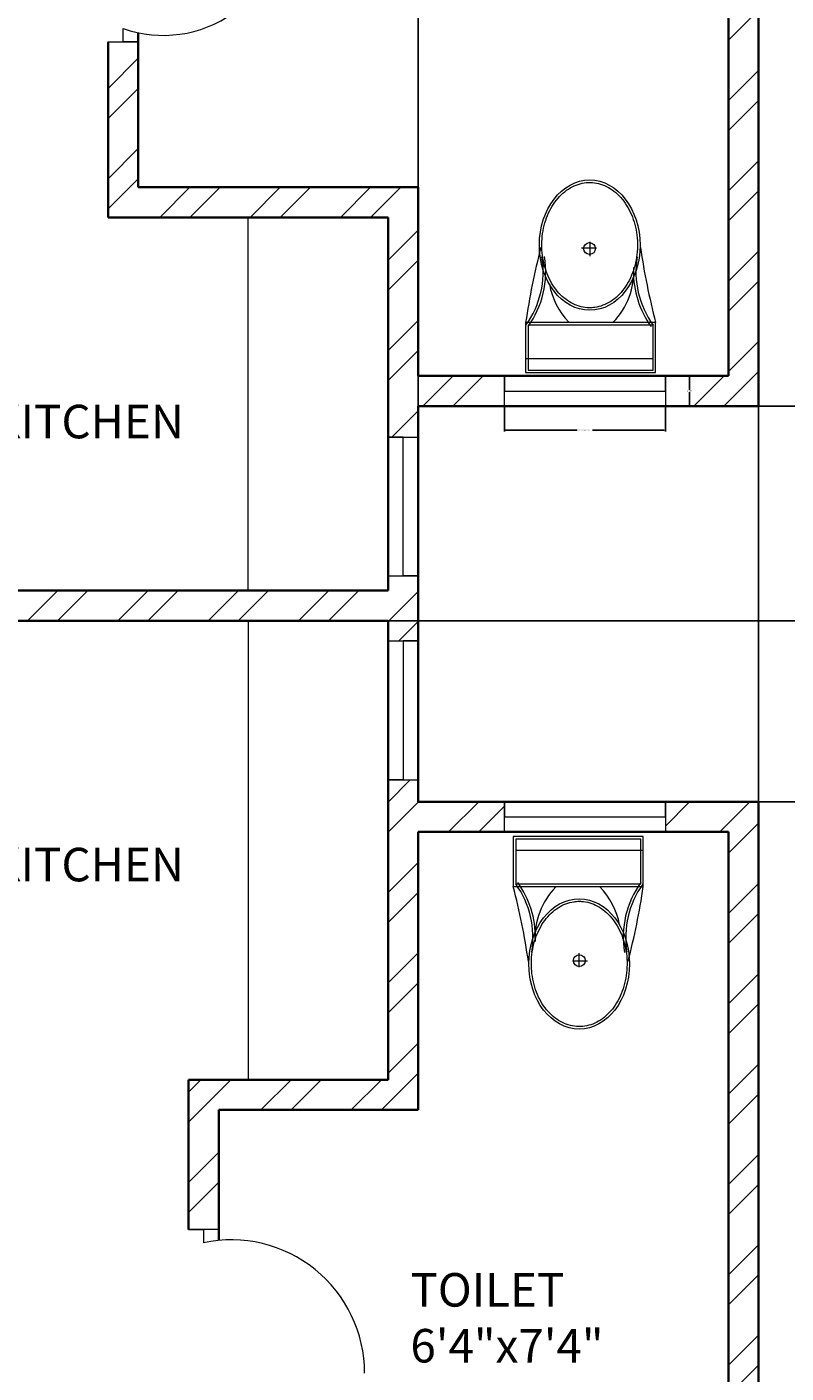
# Model space of a CAD drawing. Units: inches. Extents: x 2165 to 3042, y 1626 to 2968.
# Tile 8 of 11: x 2776 to 2889, y 1990 to 2191. Entities that reach past the tile are written whole.
import ezdxf

# ---------------------------------------------------------------- set-up
doc = ezdxf.new("R2010")
doc.units = ezdxf.units.IN
for name, color, linetype, lineweight in [('A-ANNO-DIMS', 2, 'Continuous', 18), ('A-AREA-IDEN', 7, 'Continuous', 18), ('A-DOOR', 3, 'Continuous', 18), ('A-FLOR-CASE', 8, 'Continuous', 18), ('A-FLOR-FIXT', 9, 'Continuous', 18), ('A-GLAZ', 4, 'Continuous', 18), ('A-WALL', 7, 'Continuous', 35), ('A-WALL-PATT', 252, 'Continuous', 13)]:
    doc.layers.add(name, color=color, linetype=linetype, lineweight=lineweight)
doc.styles.get("Standard").update_dxf_attribs({"font": 'arial.ttf'})
doc.dimstyles.get("Standard").update_dxf_attribs({"dimtxt": 0.18, "dimasz": 0.18, "dimexe": 0.18, "dimexo": 0.0625, "dimgap": 0.09, "dimtad": 0, "dimtih": 1, "dimtoh": 1, "dimdec": 4, "dimzin": 0, "dimdsep": 46, "dimtxsty": 'Standard', "dimcen": 0.09, "dimadec": 0, "dimazin": 0, "dimtfac": 1, "dimtdec": 4, "dimtofl": 0, "dimtmove": 0, "dimatfit": 3, "dimfxl": 1, "dimtolj": 1, "dimtzin": 0, "dimarcsym": 0})

# ---------------------------------------------------------------- blocks, each defined once
blk = doc.blocks.new('A$C31115884')
for p, q in [((283.1, 497.7), (223.4, 497.7)), ((257.5, 466.4), (257.5, 523.2)), ((0, 200), (0, 0)), ((520, 200), (0, 200)), ((10, 190), (10, 10)), ((510, 190), (10, 190)), ((510, 10), (510, 190)), ((520, 0), (520, 200)), ((510, 54.5), (0, 54.5)), ((10, 10), (510, 10)), ((0, 0), (520, 0))]:
    blk.add_line(p, q)
blk.add_circle((255.6, 496.4), 23.6)
for centre, radius, start, end in [((2777.7, -204.6), 2807, 165.4549, 171.7133), ((3237, 905), 2807, 188.2867, 194.5451), ((-294.5, 403.3), 364.7, 324.2091, 9.3499), ((-294.5, 403.3), 374.7, 324.2091, 9.3499), ((805.8, 403.3), 364.7, 170.6501, 215.7909), ((139.5, 406.2), 293.5, 315.8436, 2.6563), ((805.8, 403.3), 374.7, 179.2036, 215.7909), ((383.6, 406.2), 293.5, 190.2774, 224.1564)]:
    blk.add_arc(centre, radius, start, end)
blk.add_ellipse((256.2, 509.9), major_axis=(0, -260.7), ratio=0.772727)
blk.add_open_spline([(256.2, 259.2), (263.1, 259.2), (270, 259.7), (287.8, 262.3), (298.7, 265.1), (319.9, 273.1), (330.2, 278.4), (350.1, 291.1), (359.7, 298.7), (377.7, 315.9), (386.2, 325.5), (401.7, 346.6), (408.8, 358.1), (421.3, 382.5), (426.8, 395.5), (435.9, 422.4), (439.5, 436.4), (444.8, 465.1), (446.5, 479.7), (447.9, 509.2), (447.6, 524), (445, 553.3), (442.7, 567.8), (436.3, 596), (432.1, 609.7), (421.9, 636), (416, 648.6), (402.5, 672.1), (395, 683), (378.6, 703), (369.8, 712.1), (351.1, 728), (341.3, 734.8), (320.9, 746.2), (310.4, 750.7), (288.9, 757.3), (278, 759.4), (256, 761), (245, 760.6), (223.1, 757.2), (212.3, 754.3), (191.1, 746.1), (180.8, 740.7), (160.9, 727.8), (151.4, 720.1), (133.5, 702.7), (125.1, 693), (109.6, 671.7), (102.6, 660.2), (90.2, 635.7), (84.9, 622.7), (76, 595.6), (72.4, 581.6), (67.2, 552.9), (65.6, 538.2), (64.4, 508.8), (64.8, 494), (67.5, 464.7), (69.9, 450.2), (76.6, 422), (80.8, 408.3), (91.1, 382.2), (97.2, 369.7), (110.8, 346.3), (118.4, 335.4), (134.8, 315.6), (143.7, 306.7), (162.4, 290.9), (172.3, 284.2), (192.8, 273), (203.3, 268.6), (224.8, 262.2), (235.8, 260.2), (249.9, 259.3), (253, 259.2), (256.2, 259.2)], degree=3, knots=[0, 0, 0, 0, 0.110105, 0.110105, 0.285049, 0.285049, 0.459994, 0.459994, 0.634938, 0.634938, 0.809882, 0.809882, 0.984827, 0.984827, 1.159771, 1.159771, 1.334715, 1.334715, 1.50966, 1.50966, 1.684604, 1.684604, 1.859549, 1.859549, 2.034493, 2.034493, 2.209437, 2.209437, 2.384382, 2.384382, 2.559326, 2.559326, 2.73427, 2.73427, 2.909215, 2.909215, 3.084159, 3.084159, 3.259103, 3.259103, 3.434048, 3.434048, 3.608992, 3.608992, 3.783936, 3.783936, 3.958881, 3.958881, 4.133825, 4.133825, 4.30877, 4.30877, 4.483714, 4.483714, 4.658658, 4.658658, 4.833603, 4.833603, 5.008547, 5.008547, 5.183491, 5.183491, 5.358436, 5.358436, 5.53338, 5.53338, 5.708324, 5.708324, 5.883269, 5.883269, 6.058213, 6.058213, 6.233158, 6.233158, 6.283185, 6.283185, 6.283185, 6.283185])
blk = doc.blocks.new('WIN-24')
for p, q in [((0, 0), (0, 4.5)), ((0, 4.5), (0, 2.25)), ((24, 2.25), (24, 4.5)), ((24, 4.5), (24, 0)), ((0, 2.25), (24, 2.25))]:
    blk.add_line(p, q)
blk = doc.blocks.new('*D28')
at = {"layer": 'A-ANNO-DIMS', "color": 0, "lineweight": -2, "transparency": 16777216}
for p, q in [((2847.2, 2134.52), (2847.2, 2130.8)), ((2871.2, 2134.52), (2871.2, 2130.8)), ((2847.38, 2130.98), (2858.05, 2130.98)), ((2871.02, 2130.98), (2860.36, 2130.98))]:
    blk.add_line(p, q, dxfattribs=at)
at = {"layer": 'A-ANNO-DIMS', "color": 0, "transparency": 16777216}
for points in [[(2847.38, 2131.01), (2847.38, 2130.95), (2847.2, 2130.98)], [(2871.02, 2131.01), (2871.02, 2130.95), (2871.2, 2130.98)]]:
    blk.add_solid(points, dxfattribs=at)
at = {"layer": 'Defpoints', "color": 0, "transparency": 16777216}
for p in [(2847.2, 2134.58), (2871.2, 2134.58), (2871.2, 2130.98)]:
    blk.add_point(p, dxfattribs=at)
at = {"layer": 'A-ANNO-DIMS', "color": 0, "transparency": 16777216, "insert": (2859.2, 2130.98), "char_height": 0.18, "attachment_point": 5}
blk.add_mtext('\\A1;WC SASH 24 TYP.', dxfattribs=at)
blk = doc.blocks.new('*D29')
at = {"layer": 'A-ANNO-DIMS', "color": 0, "lineweight": -2, "transparency": 16777216}
for p, q in [((2871.27, 2139.08), (2874.98, 2139.08)), ((2874.8, 2138.9), (2874.8, 2137.01)), ((2874.8, 2134.76), (2874.8, 2136.65)), ((2871.27, 2134.58), (2874.98, 2134.58))]:
    blk.add_line(p, q, dxfattribs=at)
at = {"layer": 'A-ANNO-DIMS', "color": 0, "transparency": 16777216}
for points in [[(2874.77, 2138.9), (2874.83, 2138.9), (2874.8, 2139.08)], [(2874.77, 2134.76), (2874.83, 2134.76), (2874.8, 2134.58)]]:
    blk.add_solid(points, dxfattribs=at)
at = {"layer": 'Defpoints', "color": 0, "transparency": 16777216}
for p in [(2871.2, 2139.08), (2874.8, 2139.08), (2871.2, 2134.58)]:
    blk.add_point(p, dxfattribs=at)
at = {"layer": 'A-ANNO-DIMS', "color": 0, "transparency": 16777216, "insert": (2874.8, 2136.83), "char_height": 0.18, "attachment_point": 5}
blk.add_mtext('\\A1;5 TYP.', dxfattribs=at)
blk = doc.blocks.new('*D58')
at = {"layer": 'A-ANNO-DIMS', "color": 0, "lineweight": -2, "transparency": 16777216}
for p, q in [((2885.17, 2075.58), (2919.58, 2075.58)), ((2919.4, 2075.4), (2919.4, 2027.26)), ((2919.4, 1978.76), (2919.4, 2026.9)), ((2880.67, 1978.58), (2919.58, 1978.58))]:
    blk.add_line(p, q, dxfattribs=at)
at = {"layer": 'A-ANNO-DIMS', "color": 0, "transparency": 16777216}
for points in [[(2919.37, 2075.4), (2919.43, 2075.4), (2919.4, 2075.58)], [(2919.37, 1978.76), (2919.43, 1978.76), (2919.4, 1978.58)]]:
    blk.add_solid(points, dxfattribs=at)
at = {"layer": 'Defpoints', "color": 0, "transparency": 16777216}
for p in [(2885.1, 2075.58), (2919.4, 2075.58), (2880.6, 1978.58)]:
    blk.add_point(p, dxfattribs=at)
at = {"layer": 'A-ANNO-DIMS', "color": 0, "transparency": 16777216, "insert": (2919.4, 2027.08), "char_height": 0.18, "attachment_point": 5}
blk.add_mtext('\\A1;97', dxfattribs=at)
blk = doc.blocks.new('*D59')
at = {"layer": 'A-ANNO-DIMS', "color": 0, "lineweight": -2, "transparency": 16777216}
for p, q in [((2829.92, 2102.58), (2919.58, 2102.58)), ((2919.4, 2102.4), (2919.4, 2089.26)), ((2919.4, 2075.76), (2919.4, 2088.9)), ((2885.17, 2075.58), (2919.58, 2075.58))]:
    blk.add_line(p, q, dxfattribs=at)
at = {"layer": 'A-ANNO-DIMS', "color": 0, "transparency": 16777216}
for points in [[(2919.37, 2102.4), (2919.43, 2102.4), (2919.4, 2102.58)], [(2919.37, 2075.76), (2919.43, 2075.76), (2919.4, 2075.58)]]:
    blk.add_solid(points, dxfattribs=at)
at = {"layer": 'Defpoints', "color": 0, "transparency": 16777216}
for p in [(2829.85, 2102.58), (2919.4, 2102.58), (2885.1, 2075.58)]:
    blk.add_point(p, dxfattribs=at)
at = {"layer": 'A-ANNO-DIMS', "color": 0, "transparency": 16777216, "insert": (2919.4, 2089.08), "char_height": 0.18, "attachment_point": 5}
blk.add_mtext('\\A1;27', dxfattribs=at)
blk = doc.blocks.new('*D60')
at = {"layer": 'A-ANNO-DIMS', "color": 0, "lineweight": -2, "transparency": 16777216}
for p, q in [((2885.17, 2134.58), (2919.58, 2134.58)), ((2919.4, 2134.4), (2919.4, 2118.76)), ((2919.4, 2102.76), (2919.4, 2118.4)), ((2829.92, 2102.58), (2919.58, 2102.58))]:
    blk.add_line(p, q, dxfattribs=at)
at = {"layer": 'A-ANNO-DIMS', "color": 0, "transparency": 16777216}
for points in [[(2919.37, 2134.4), (2919.43, 2134.4), (2919.4, 2134.58)], [(2919.37, 2102.76), (2919.43, 2102.76), (2919.4, 2102.58)]]:
    blk.add_solid(points, dxfattribs=at)
at = {"layer": 'Defpoints', "color": 0, "transparency": 16777216}
for p in [(2885.1, 2134.58), (2919.4, 2134.58), (2829.85, 2102.58)]:
    blk.add_point(p, dxfattribs=at)
at = {"layer": 'A-ANNO-DIMS', "color": 0, "transparency": 16777216, "insert": (2919.4, 2118.58), "char_height": 0.18, "attachment_point": 5}
blk.add_mtext('\\A1;32', dxfattribs=at)
blk = doc.blocks.new('*D61')
at = {"layer": 'A-ANNO-DIMS', "color": 0, "lineweight": -2, "transparency": 16777216}
for p, q in [((2880.67, 2215.08), (2919.58, 2215.08)), ((2919.4, 2214.9), (2919.4, 2175.01)), ((2919.4, 2134.76), (2919.4, 2174.65)), ((2885.17, 2134.58), (2919.58, 2134.58))]:
    blk.add_line(p, q, dxfattribs=at)
at = {"layer": 'A-ANNO-DIMS', "color": 0, "transparency": 16777216}
for points in [[(2919.37, 2214.9), (2919.43, 2214.9), (2919.4, 2215.08)], [(2919.37, 2134.76), (2919.43, 2134.76), (2919.4, 2134.58)]]:
    blk.add_solid(points, dxfattribs=at)
at = {"layer": 'Defpoints', "color": 0, "transparency": 16777216}
for p in [(2880.6, 2215.08), (2919.4, 2215.08), (2885.1, 2134.58)]:
    blk.add_point(p, dxfattribs=at)
at = {"layer": 'A-ANNO-DIMS', "color": 0, "transparency": 16777216, "insert": (2919.4, 2174.83), "char_height": 0.18, "attachment_point": 5}
blk.add_mtext('\\A1;80.5', dxfattribs=at)
blk = doc.blocks.new('*D63')
at = {"layer": 'A-ANNO-DIMS', "color": 0, "lineweight": -2, "transparency": 16777216}
for p, q in [((2834.35, 2075.64), (2834.35, 2398.06)), ((2834.53, 2397.88), (2859.34, 2397.88)), ((2884.92, 2397.88), (2860.12, 2397.88)), ((2885.1, 2075.64), (2885.1, 2398.06))]:
    blk.add_line(p, q, dxfattribs=at)
at = {"layer": 'A-ANNO-DIMS', "color": 0, "transparency": 16777216}
for points in [[(2834.53, 2397.91), (2834.53, 2397.85), (2834.35, 2397.88)], [(2884.92, 2397.91), (2884.92, 2397.85), (2885.1, 2397.88)]]:
    blk.add_solid(points, dxfattribs=at)
at = {"layer": 'Defpoints', "color": 0, "transparency": 16777216}
for p in [(2885.1, 2397.88), (2834.35, 2075.58), (2885.1, 2075.58)]:
    blk.add_point(p, dxfattribs=at)
at = {"layer": 'A-ANNO-DIMS', "color": 0, "transparency": 16777216, "insert": (2859.73, 2397.88), "char_height": 0.18, "attachment_point": 5}
blk.add_mtext('\\A1;50.75', dxfattribs=at)

msp = doc.modelspace()

# ---------------------------------------------------------------- hatches: boundary and pattern name
at = {"layer": 'A-WALL-PATT'}
h = msp.add_hatch(dxfattribs=at)
h.set_pattern_fill('ANSI32', color=256)
h.paths.add_polyline_path([(2406.4931, 2332.0783), (2286.6045, 2332.0783), (2286.6045, 2310.967), (2288.8545, 2310.967), (2291.1045, 2310.967), (2291.1045, 2327.5783), (2406.4931, 2327.5783), (2406.4931, 2329.8283)])
h.paths.add_polyline_path([(2439.6045, 2327.5783), (2444.9584, 2327.5783), (2444.9584, 2332.0783), (2430.2901, 2332.0783), (2430.2901, 2329.8283), (2430.2901, 2327.5783), (2435.1045, 2327.5783), (2435.1045, 2219.5783), (2431.0902, 2219.5783), (2431.0902, 2215.0783), (2435.1045, 2215.0783), (2444.1108, 2215.0783), (2444.1108, 2217.3283), (2444.1108, 2219.5783), (2439.6045, 2219.5783)])
h.paths.add_polyline_path([(2497.5418, 2329.8283), (2497.5418, 2332.0783), (2470.1978, 2332.0783), (2470.1978, 2327.5783), (2497.5418, 2327.5783)])
h.paths.add_polyline_path([(2617.9543, 2332.0783), (2557.5418, 2332.0783), (2557.5418, 2327.5783), (2583.6045, 2327.5783), (2583.6045, 2219.5783), (2474.0523, 2219.5783), (2474.0523, 2215.0783), (2583.6045, 2215.0783), (2583.6045, 2107.0783), (2579.3609, 2107.0783), (2579.3609, 2102.5783), (2588.1045, 2102.5783), (2593.5283, 2102.5783), (2593.5283, 2104.8283), (2593.5283, 2107.0783), (2588.1045, 2107.0783), (2588.1045, 2215.0783), (2691.2325, 2215.0783), (2691.2325, 2217.3283), (2691.2325, 2219.5783), (2588.1045, 2219.5783), (2588.1045, 2327.5783), (2617.9543, 2327.5783)])
h.paths.add_polyline_path([(2702.4444, 2329.8283), (2702.4444, 2332.0783), (2677.9543, 2332.0783), (2677.9543, 2327.5783), (2702.4444, 2327.5783)])
h.paths.add_polyline_path([(2736.6045, 2327.5783), (2742.5161, 2327.5783), (2742.5161, 2329.8283), (2742.5161, 2332.0783), (2727.7639, 2332.0783), (2727.7639, 2329.8283), (2727.7639, 2327.5783), (2732.1045, 2327.5783), (2732.1045, 2219.5783), (2726.4404, 2219.5783), (2726.4404, 2215.0783), (2732.1045, 2215.0783), (2742.7291, 2215.0783), (2742.7291, 2217.3283), (2742.7291, 2219.5783), (2736.6045, 2219.5783)])
h.paths.add_polyline_path([(2885.1045, 2332.0783), (2768.4887, 2332.0783), (2768.4887, 2327.5783), (2784.6045, 2327.5783), (2880.6045, 2327.5783), (2880.6045, 2310.967), (2885.1045, 2310.967)])
h.paths.add_polyline_path([(2885.1045, 2250.967), (2880.6045, 2250.967), (2880.6045, 2219.5783), (2776.5755, 2219.5783), (2776.5755, 2215.0783), (2788.1045, 2215.0783), (2788.1045, 2209.8634), (2790.3545, 2209.8634), (2792.6045, 2209.8634), (2792.6045, 2215.0783), (2880.6045, 2215.0783), (2880.6045, 2139.0783), (2871.2037, 2139.0783), (2871.2037, 2134.5783), (2885.1045, 2134.5783)])
h.paths.add_polyline_path([(2545.013, 2107.0783), (2474.0523, 2107.0783), (2291.1045, 2107.0783), (2291.1045, 2102.5783), (2535.6045, 2102.5783), (2535.6045, 2096.8046), (2537.8545, 2096.8046), (2540.1045, 2096.8046), (2540.1045, 2102.5783), (2545.013, 2102.5783), (2545.013, 2104.8283)])
h.paths.add_polyline_path([(2397.7297, 2217.3283), (2397.7297, 2219.5783), (2291.1045, 2219.5783), (2291.1045, 2250.967), (2286.6045, 2250.967), (2286.6045, 2206.1346), (2288.8545, 2206.1346), (2291.1045, 2206.1346), (2291.1045, 2215.0783), (2367.1045, 2215.0783), (2367.1045, 2212.2868), (2371.6045, 2212.2868), (2371.6045, 2215.0783), (2397.7297, 2215.0783)])
h.paths.add_polyline_path([(2291.1045, 1978.5783), (2367.1045, 1978.5783), (2371.6045, 1978.5783), (2373.2641, 1978.5783), (2374.4883, 1978.5783), (2374.4883, 1980.8283), (2374.4883, 1983.0783), (2371.6045, 1983.0783), (2371.6045, 1986.964), (2369.9051, 1986.964), (2369.3545, 1986.964), (2367.1045, 1986.964), (2367.1045, 1983.0783), (2291.1045, 1983.0783), (2291.1045, 2001.1808), (2286.6045, 2001.1808), (2286.6045, 1947.0203), (2288.8545, 1947.0203), (2291.1045, 1947.0203)])
h.paths.add_polyline_path([(2291.1045, 1887.0203), (2286.6045, 1887.0203), (2286.6045, 1842.0783), (2381.2561, 1842.0783), (2381.2561, 1844.3283), (2381.2561, 1846.5783), (2363.1045, 1846.5783), (2291.1045, 1846.5783)])
h.paths.add_polyline_path([(2415.6045, 1978.5783), (2421.1681, 1978.5783), (2421.1681, 1983.0783), (2415.6045, 1983.0783), (2406.5227, 1983.0783), (2406.5227, 1980.8283), (2406.5227, 1978.5783), (2411.1045, 1978.5783), (2411.1045, 1846.5783), (2406.7549, 1846.5783), (2406.7549, 1842.0783), (2419.2885, 1842.0783), (2419.2885, 1844.3283), (2419.2885, 1846.5783), (2415.6045, 1846.5783)])
h.paths.add_polyline_path([(2586.6045, 1982.779), (2586.6045, 1991.5911), (2582.1045, 1991.5911), (2582.1045, 1982.779), (2540.1045, 1982.779), (2540.1045, 2036.779), (2582.1045, 2036.779), (2582.1045, 2027.6051), (2586.6045, 2027.6051), (2586.6045, 2041.279), (2582.1045, 2041.279), (2540.1045, 2041.279), (2540.1045, 2063.9064), (2537.8545, 2063.9064), (2535.6045, 2063.9064), (2535.6045, 1983.0783), (2455.068, 1983.0783), (2455.068, 1978.5783), (2535.6045, 1978.5783), (2535.6045, 1846.5783), (2522.622, 1846.5783), (2522.622, 1842.0783), (2535.6045, 1842.0783), (2535.6045, 1806.0783), (2535.6045, 1801.5783), (2556.726, 1801.5783), (2556.726, 1803.8283), (2556.726, 1806.0783), (2540.1045, 1806.0783), (2540.1045, 1842.0783), (2540.1045, 1846.5783), (2540.1045, 1978.279), (2586.6045, 1978.279)])
h.paths.add_polyline_path([(2636.1045, 1978.5783), (2717.6642, 1978.5783), (2717.6642, 1980.8283), (2717.6642, 1983.0783), (2636.1045, 1983.0783), (2636.1045, 2063.9064), (2633.8545, 2063.9064), (2631.6045, 2063.9064), (2631.6045, 1846.5783), (2631.6045, 1842.0783), (2631.6045, 1806.0783), (2604.726, 1806.0783), (2604.726, 1801.5783), (2636.1045, 1801.5783), (2636.1045, 1842.0783), (2644.3411, 1842.0783), (2644.3411, 1844.3283), (2644.3411, 1846.5783), (2636.1045, 1846.5783)])
h.paths.add_polyline_path([(2760.6045, 1978.5783), (2764.9931, 1978.5783), (2764.9931, 1983.0783), (2750.4727, 1983.0783), (2750.4727, 1980.8283), (2750.4727, 1978.5783), (2756.1045, 1978.5783), (2756.1045, 1846.5783), (2749.4543, 1846.5783), (2749.4543, 1842.0783), (2765.1894, 1842.0783), (2765.1894, 1846.5783), (2760.6045, 1846.5783)])
h.paths.add_polyline_path([(2880.6045, 1983.0783), (2804.6045, 1983.0783), (2804.6045, 1988.3825), (2802.3545, 1988.3825), (2800.1045, 1988.3825), (2800.1045, 1983.0783), (2800.1045, 1978.5783), (2880.6045, 1978.5783)])
h.paths.add_polyline_path([(2885.1045, 2075.5783), (2871.2037, 2075.5783), (2871.2037, 2071.0783), (2880.6045, 2071.0783), (2880.6045, 1948.8144), (2885.1045, 1948.8144)])
h.paths.add_polyline_path([(2885.1045, 1888.8144), (2880.6045, 1888.8144), (2880.6045, 1846.5783), (2792.1167, 1846.5783), (2792.1167, 1842.0783), (2885.1045, 1842.0783)])
h.paths.add_polyline_path([(2724.4848, 1846.5783), (2708.1045, 1846.5783), (2692.3411, 1846.5783), (2692.3411, 1842.0783), (2724.4848, 1842.0783), (2724.4848, 1844.3283)])
h.paths.add_polyline_path([(2474.622, 1844.4672), (2474.622, 1846.5783), (2444.7417, 1846.5783), (2444.7417, 1842.0783), (2474.622, 1842.0783)])
h = msp.add_hatch(dxfattribs=at)
h.set_pattern_fill('ANSI32', color=256)
h.paths.add_polyline_path([(2834.3545, 2109.2607), (2832.1045, 2109.2607), (2829.8545, 2109.2607), (2829.8545, 2107.0783), (2788.1045, 2107.0783), (2627.8367, 2107.0783), (2627.8367, 2102.5783), (2631.6045, 2102.5783), (2631.6045, 2096.8046), (2636.1045, 2096.8046), (2636.1045, 2102.5783), (2788.1045, 2102.5783), (2829.8545, 2102.5783), (2829.8545, 2099.5599), (2834.3545, 2099.5599), (2834.3545, 2102.5783)])
h.paths.add_polyline_path([(2834.3545, 2162.7002), (2834.3545, 2167.2002), (2792.6045, 2167.2002), (2792.6045, 2188.8893), (2790.3545, 2188.8893), (2788.1045, 2188.8893), (2788.1045, 2162.7002), (2829.8545, 2162.7002), (2829.8545, 2134.5783), (2829.8545, 2129.9534), (2834.3545, 2129.9534), (2834.3545, 2134.5783), (2847.2037, 2134.5783), (2847.2037, 2139.0783), (2834.3545, 2139.0783)])
h.paths.add_polyline_path([(2834.3545, 2071.0783), (2847.2037, 2071.0783), (2847.2037, 2075.5783), (2834.3545, 2075.5783), (2834.3545, 2078.8214), (2829.8545, 2078.8214), (2829.8545, 2075.5783), (2829.8545, 2034.1177), (2800.1045, 2034.1177), (2800.1045, 2011.8162), (2802.3375, 2011.8162), (2804.6045, 2011.8162), (2804.6045, 2029.6177), (2834.3545, 2029.6177), (2834.3545, 2034.1177)])

# ---------------------------------------------------------------- linework, layer by layer
at = {"layer": 'A-DOOR'}
for p, q in [((2790.3545, 2188.8893), (2790.3545, 2190.8893)), ((2788.1045, 2188.8893), (2792.6045, 2188.8893)), ((2792.6045, 2188.8893), (2790.3545, 2188.8893)), ((2790.3545, 2188.8893), (2790.3545, 2188.8893)), ((2801.4524, 2011.8162), (2800.1045, 2011.8162)), ((2800.1045, 2011.8162), (2802.3375, 2011.8162)), ((2804.6045, 2011.8162), (2801.4524, 2011.8162)), ((2802.3375, 2011.8162), (2802.3375, 2009.8162))]:
    msp.add_line(p, q, dxfattribs=at)
for centre, radius, start, end in [((2796.3519, 2207.8634), 18.0025, 250.540061, 0), ((2806.4834, 1990.3825), 19.8711, 0, 102.042606)]:
    msp.add_arc(centre, radius, start, end, dxfattribs=at)
at = {"layer": 'A-FLOR-CASE'}
for p, q in [((2808.9795, 2107.0783), (2808.9795, 2162.7002)), ((2808.9795, 2102.5783), (2808.9795, 2034.1177))]:
    msp.add_line(p, q, dxfattribs=at)
at = {"layer": 'A-GLAZ'}
for p, q in [((2832.1045, 2129.9534), (2829.8545, 2129.9534)), ((2829.8545, 2129.9534), (2834.3545, 2129.9534)), ((2832.1045, 2109.2607), (2832.1045, 2129.9534)), ((2829.8545, 2109.2607), (2834.3545, 2109.2607)), ((2834.3545, 2109.2607), (2832.1045, 2109.2607)), ((2829.8545, 2099.5599), (2834.3545, 2099.5599)), ((2834.3545, 2099.5599), (2832.1045, 2099.5599)), ((2832.1045, 2099.5599), (2832.1045, 2078.8214)), ((2832.1045, 2078.8214), (2829.8545, 2078.8214)), ((2829.8545, 2078.8214), (2834.3545, 2078.8214))]:
    msp.add_line(p, q, dxfattribs=at)
at = {"layer": 'A-WALL'}
for p, q in [((2885.1045, 2332.0783), (2885.1045, 2134.5783)), ((2880.6045, 2215.0783), (2880.6045, 2139.0783)), ((2792.6045, 2190.2552), (2792.6045, 2167.2002)), ((2788.1045, 2188.8893), (2788.1045, 2162.7002)), ((2834.3545, 2167.2002), (2792.6045, 2167.2002)), ((2834.3545, 2162.7002), (2834.3545, 2167.2002)), ((2829.8545, 2162.7002), (2788.1045, 2162.7002)), ((2829.8545, 2134.5783), (2829.8545, 2162.7002)), ((2834.3545, 2139.0783), (2834.3545, 2162.7002)), ((2834.3545, 2139.0783), (2880.6045, 2139.0783)), ((2829.8545, 2107.0783), (2829.8545, 2134.5783)), ((2834.3545, 2134.5783), (2885.1045, 2134.5783)), ((2834.3545, 2134.5783), (2834.3545, 2075.5783)), ((2834.3545, 2134.5783), (2834.3545, 2134.5783)), ((2626.1408, 2107.0783), (2788.1045, 2107.0783)), ((2788.1045, 2107.0783), (2829.8545, 2107.0783)), ((2636.1045, 2102.5783), (2788.1045, 2102.5783)), ((2788.1045, 2102.5783), (2829.8545, 2102.5783)), ((2829.8545, 2075.5783), (2829.8545, 2102.5783)), ((2834.3545, 2102.5783), (2834.3545, 2075.5783)), ((2829.8545, 2075.5783), (2829.8545, 2034.1177)), ((2834.3545, 2075.5783), (2885.1045, 2075.5783)), ((2885.1045, 2075.5783), (2885.1045, 1842.0783)), ((2834.3545, 2071.0783), (2880.6045, 2071.0783)), ((2834.3545, 2071.0783), (2834.3545, 2034.1177)), ((2880.6045, 2071.0783), (2880.6045, 1846.5783)), ((2800.1045, 2034.1177), (2800.1045, 2011.8162)), ((2829.8545, 2034.1177), (2800.1045, 2034.1177)), ((2834.3545, 2034.1177), (2834.3545, 2029.6177)), ((2834.3545, 2029.6177), (2804.6045, 2029.6177)), ((2804.6045, 2029.6177), (2804.6045, 2010.1645))]:
    msp.add_line(p, q, dxfattribs=at)

# ---------------------------------------------------------------- block references
at = {"layer": 'A-FLOR-FIXT', "xscale": 0.0372717239612423, "yscale": 0.0372717239612423, "zscale": 0.0372717239612423}
msp.add_blockref('A$C31115884', (2850.3711, 2139.5741), dxfattribs=at)
at = {"layer": 'A-FLOR-FIXT', "xscale": 0.0372717239612423, "yscale": 0.0372717239612423, "zscale": 0.0372717239612423, "rotation": 180}
msp.add_blockref('A$C31115884', (2867.9022, 2070.3952), dxfattribs=at)
at = {"layer": 'A-GLAZ'}
for p in [(2847.204, 2134.578), (2847.204, 2071.078)]:
    msp.add_blockref('WIN-24', p, dxfattribs=at)

# ---------------------------------------------------------------- texts
at = {"layer": 'A-AREA-IDEN', "char_height": 5, "attachment_point": 1}
for s, width, insert in [('KITCHEN', 171.28889, (2770.6672, 2134.7728)), ('KITCHEN', 171.28889, (2770.6672, 2068.7105)), ('TOILET\\P6\'4"x7\'4"', 94.381891, (2833.1893, 2005.2944))]:
    msp.add_mtext_dynamic_manual_height_columns(s, width=width, gutter_width=12.5, heights=[0], dxfattribs=dict(at, insert=insert))

# ---------------------------------------------------------------- dimensions: what is measured, and where the dimension line sits
at = {"layer": 'A-ANNO-DIMS'}
dim = msp.add_linear_dim(base=(2885.1045, 2397.8783), p1=(2834.3545, 2075.5783), p2=(2885.1045, 2075.5783), dimstyle='Standard', override={"dimdec": 2, "dimlfac": 1, "dimrnd": 0, "dimzin": 0, "dimdsep": 46, "dimlunit": 2}, dxfattribs=at)
dim.commit()
dim.dimension.update_dxf_attribs({"geometry": '*D63', "text_midpoint": (2859.7295, 2397.8783)})
for base, p1, p2, override, picture, middle in [((2919.4045, 2215.0783), (2885.1045, 2134.5783), (2880.6045, 2215.0783), {"dimdec": 1, "dimlfac": 1, "dimrnd": 0, "dimzin": 0, "dimdsep": 46, "dimlunit": 2}, '*D61', (2919.4045, 2174.8283)), ((2919.4045, 2134.5783), (2829.8545, 2102.5783), (2885.1045, 2134.5783), {"dimdec": 0, "dimlfac": 1, "dimrnd": 0, "dimzin": 0, "dimdsep": 46, "dimlunit": 2}, '*D60', (2919.4045, 2118.5783)), ((2919.4045, 2102.5783), (2885.1045, 2075.5783), (2829.8545, 2102.5783), {"dimdec": 0, "dimlfac": 1, "dimrnd": 0, "dimzin": 0, "dimdsep": 46, "dimlunit": 2}, '*D59', (2919.4045, 2089.0783)), ((2919.4045, 2075.5783), (2880.6045, 1978.5783), (2885.1045, 2075.5783), {"dimdec": 0, "dimlfac": 1, "dimrnd": 0, "dimzin": 0, "dimdsep": 46, "dimlunit": 2}, '*D58', (2919.4045, 2027.0783))]:
    dim = msp.add_linear_dim(base=base, p1=p1, p2=p2, angle=90, dimstyle='Standard', override=override, dxfattribs=at)
    dim.commit()
    dim.dimension.update_dxf_attribs({"geometry": picture, "text_midpoint": middle})
dim = msp.add_linear_dim(base=(2874.8036618047, 2139.0783076613), p1=(2871.2036618047, 2134.5783076613), p2=(2871.2036618047, 2139.0783076613), angle=90, text='<> TYP.', dimstyle='Standard', override={"dimdec": 0, "dimlfac": 1, "dimrnd": 0, "dimzin": 0, "dimdsep": 46, "dimlunit": 2}, dxfattribs=at)
dim.commit()
dim.dimension.update_dxf_attribs({"geometry": '*D29', "text_midpoint": (2874.8036618047, 2136.8283076613)})
dim = msp.add_linear_dim(base=(2871.2037, 2130.9783), p1=(2847.2037, 2134.5783), p2=(2871.2037, 2134.5783), text='WC SASH <> TYP.', dimstyle='Standard', override={"dimdec": 0, "dimlfac": 1, "dimrnd": 0, "dimzin": 0, "dimdsep": 46, "dimlunit": 2}, dxfattribs=at)
dim.commit()
dim.dimension.update_dxf_attribs({"geometry": '*D28', "text_midpoint": (2859.2037, 2130.9783)})

doc.saveas('drawing.dxf')
